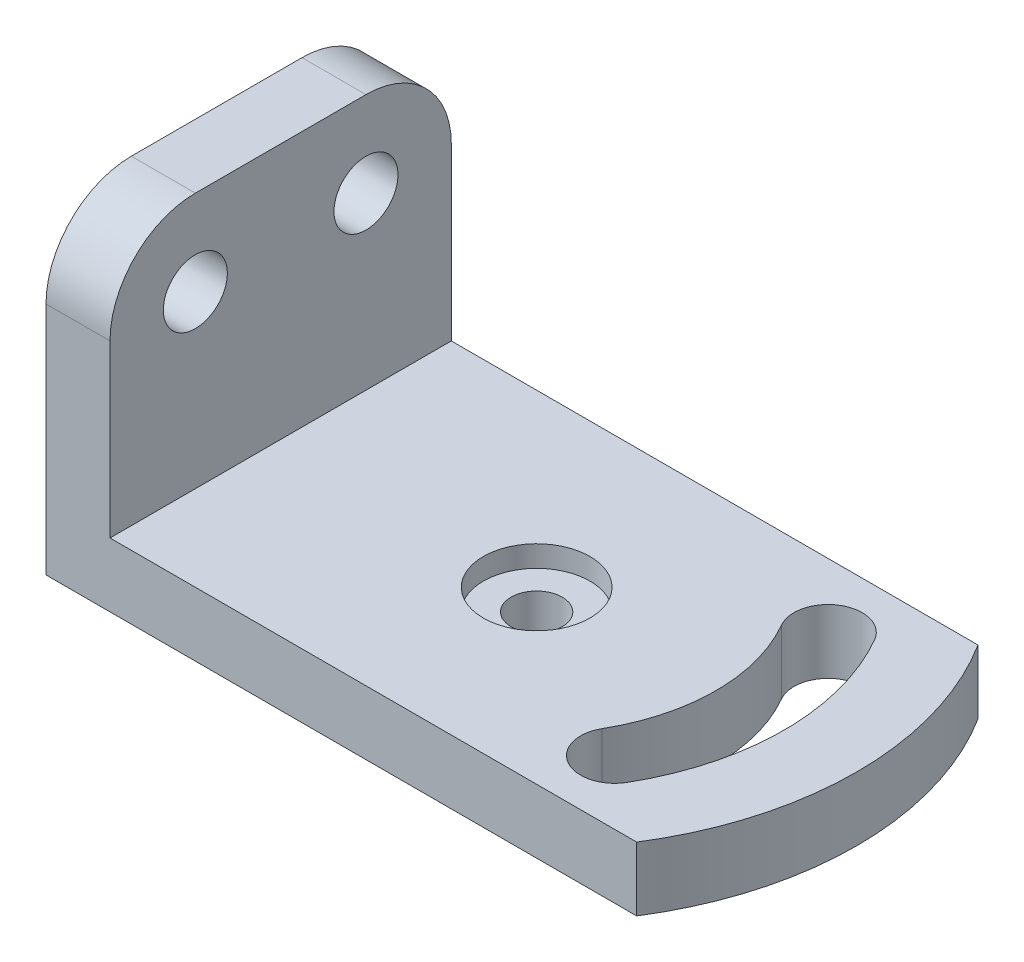
ISO-10303-21;
HEADER;
FILE_DESCRIPTION(('STEP AP214'),'2;1');
FILE_NAME('part.step','',(''),(''),'','','');
FILE_SCHEMA(('AUTOMOTIVE_DESIGN { 1 0 10303 214 1 1 1 1 }'));
ENDSEC;
DATA;
#1=APPLICATION_CONTEXT('core data for automotive mechanical design processes');
#2=APPLICATION_PROTOCOL_DEFINITION('international standard','automotive_design',2000,#1);
#3=PRODUCT_CONTEXT('',#1,'mechanical');
#4=PRODUCT('Part','Part','',(#3));
#5=PRODUCT_RELATED_PRODUCT_CATEGORY('part','',(#4));
#6=PRODUCT_DEFINITION_FORMATION('','',#4);
#7=PRODUCT_DEFINITION_CONTEXT('part definition',#1,'design');
#8=PRODUCT_DEFINITION('design','',#6,#7);
#9=PRODUCT_DEFINITION_SHAPE('','',#8);
#10=(LENGTH_UNIT() NAMED_UNIT(*) SI_UNIT(.MILLI.,.METRE.));
#11=(NAMED_UNIT(*) PLANE_ANGLE_UNIT() SI_UNIT($,.RADIAN.));
#12=(NAMED_UNIT(*) SI_UNIT($,.STERADIAN.) SOLID_ANGLE_UNIT());
#13=UNCERTAINTY_MEASURE_WITH_UNIT(LENGTH_MEASURE(1.E-05),#10,'distance_accuracy_value','');
#14=(GEOMETRIC_REPRESENTATION_CONTEXT(3) GLOBAL_UNCERTAINTY_ASSIGNED_CONTEXT((#13)) GLOBAL_UNIT_ASSIGNED_CONTEXT((#10,
#11,#12)) REPRESENTATION_CONTEXT('',''));
#15=CARTESIAN_POINT('',(0.,0.,0.));
#16=DIRECTION('',(0.,0.,1.));
#17=DIRECTION('',(1.,0.,0.));
#18=AXIS2_PLACEMENT_3D('',#15,#16,#17);
#19=CARTESIAN_POINT('',(0.,15.,0.));
#20=DIRECTION('',(0.,1.,0.));
#21=DIRECTION('',(0.,0.,1.));
#22=AXIS2_PLACEMENT_3D('',#19,#20,#21);
#23=PLANE('',#22);
#24=CARTESIAN_POINT('',(43.3012701892219,15.,25.0000000000001));
#25=DIRECTION('',(0.,1.,0.));
#26=DIRECTION('',(0.,0.,1.));
#27=AXIS2_PLACEMENT_3D('',#24,#25,#26);
#28=CIRCLE('',#27,7.99999999999999);
#29=CARTESIAN_POINT('',(36.3730669589464,15.,21.));
#30=VERTEX_POINT('',#29);
#31=CARTESIAN_POINT('',(50.2294734194974,15.,29.0000000000001));
#32=VERTEX_POINT('',#31);
#33=EDGE_CURVE('E61',#30,#32,#28,.T.);
#34=ORIENTED_EDGE('',*,*,#33,.F.);
#35=CARTESIAN_POINT('',(0.,15.,0.));
#36=DIRECTION('',(0.,1.,0.));
#37=DIRECTION('',(0.,0.,1.));
#38=AXIS2_PLACEMENT_3D('',#35,#36,#37);
#39=CIRCLE('',#38,42.);
#40=CARTESIAN_POINT('',(36.3730669589464,15.,-21.0000000000001));
#41=VERTEX_POINT('',#40);
#42=EDGE_CURVE('E182',#30,#41,#39,.T.);
#43=ORIENTED_EDGE('',*,*,#42,.T.);
#44=CARTESIAN_POINT('',(43.3012701892219,15.,-25.0000000000001));
#45=DIRECTION('',(0.,1.,0.));
#46=DIRECTION('',(0.,0.,1.));
#47=AXIS2_PLACEMENT_3D('',#44,#45,#46);
#48=CIRCLE('',#47,7.99999999999999);
#49=CARTESIAN_POINT('',(50.2294734194974,15.,-29.0000000000001));
#50=VERTEX_POINT('',#49);
#51=EDGE_CURVE('E179',#50,#41,#48,.T.);
#52=ORIENTED_EDGE('',*,*,#51,.F.);
#53=CARTESIAN_POINT('',(0.,15.,0.));
#54=DIRECTION('',(0.,1.,0.));
#55=DIRECTION('',(0.,0.,1.));
#56=AXIS2_PLACEMENT_3D('',#53,#54,#55);
#57=CIRCLE('',#56,58.);
#58=EDGE_CURVE('E180',#32,#50,#57,.T.);
#59=ORIENTED_EDGE('',*,*,#58,.F.);
#60=EDGE_LOOP('',(#34,#43,#52,#59));
#61=FACE_BOUND('',#60,.T.);
#62=CARTESIAN_POINT('',(0.,15.,0.));
#63=DIRECTION('',(0.,1.,0.));
#64=DIRECTION('',(0.,0.,1.));
#65=AXIS2_PLACEMENT_3D('',#62,#63,#64);
#66=CIRCLE('',#65,12.5);
#67=CARTESIAN_POINT('',(0.,15.,12.5));
#68=VERTEX_POINT('',#67);
#69=EDGE_CURVE('E212',#68,#68,#66,.T.);
#70=ORIENTED_EDGE('',*,*,#69,.F.);
#71=EDGE_LOOP('',(#70));
#72=FACE_BOUND('',#71,.T.);
#73=DIRECTION('',(-1.,0.,0.));
#74=VECTOR('',#73,1.);
#75=CARTESIAN_POINT('',(-75.,15.,-40.));
#76=LINE('',#75,#74);
#77=CARTESIAN_POINT('',(63.4428877022476,15.,-40.));
#78=VERTEX_POINT('',#77);
#79=CARTESIAN_POINT('',(-60.,15.,-40.));
#80=VERTEX_POINT('',#79);
#81=EDGE_CURVE('E228',#78,#80,#76,.T.);
#82=ORIENTED_EDGE('',*,*,#81,.T.);
#83=DIRECTION('',(0.,0.,1.));
#84=VECTOR('',#83,1.);
#85=CARTESIAN_POINT('',(-60.,15.,-40.));
#86=LINE('',#85,#84);
#87=CARTESIAN_POINT('',(-60.,15.,40.));
#88=VERTEX_POINT('',#87);
#89=EDGE_CURVE('E165',#80,#88,#86,.T.);
#90=ORIENTED_EDGE('',*,*,#89,.T.);
#91=DIRECTION('',(1.,0.,0.));
#92=VECTOR('',#91,1.);
#93=CARTESIAN_POINT('',(-75.,15.,40.));
#94=LINE('',#93,#92);
#95=CARTESIAN_POINT('',(63.4428877022476,15.,40.));
#96=VERTEX_POINT('',#95);
#97=EDGE_CURVE('E230',#88,#96,#94,.T.);
#98=ORIENTED_EDGE('',*,*,#97,.T.);
#99=CARTESIAN_POINT('',(0.,15.,0.));
#100=DIRECTION('',(0.,1.,0.));
#101=DIRECTION('',(0.,0.,1.));
#102=AXIS2_PLACEMENT_3D('',#99,#100,#101);
#103=CIRCLE('',#102,75.);
#104=EDGE_CURVE('E217',#96,#78,#103,.T.);
#105=ORIENTED_EDGE('',*,*,#104,.T.);
#106=EDGE_LOOP('',(#82,#90,#98,#105));
#107=FACE_BOUND('',#106,.T.);
#108=ADVANCED_FACE('F41',(#61,#72,#107),#23,.T.);
#109=CARTESIAN_POINT('',(0.,0.,0.));
#110=DIRECTION('',(0.,1.,0.));
#111=DIRECTION('',(0.,0.,1.));
#112=AXIS2_PLACEMENT_3D('',#109,#110,#111);
#113=PLANE('',#112);
#114=CARTESIAN_POINT('',(0.,0.,0.));
#115=DIRECTION('',(0.,1.,0.));
#116=DIRECTION('',(0.,0.,1.));
#117=AXIS2_PLACEMENT_3D('',#114,#115,#116);
#118=CIRCLE('',#117,42.);
#119=CARTESIAN_POINT('',(36.3730669589464,0.,21.));
#120=VERTEX_POINT('',#119);
#121=CARTESIAN_POINT('',(36.3730669589464,0.,-21.0000000000001));
#122=VERTEX_POINT('',#121);
#123=EDGE_CURVE('E193',#120,#122,#118,.T.);
#124=ORIENTED_EDGE('',*,*,#123,.F.);
#125=CARTESIAN_POINT('',(43.3012701892219,0.,25.0000000000001));
#126=DIRECTION('',(0.,1.,0.));
#127=DIRECTION('',(0.,0.,1.));
#128=AXIS2_PLACEMENT_3D('',#125,#126,#127);
#129=CIRCLE('',#128,7.99999999999999);
#130=CARTESIAN_POINT('',(50.2294734194974,0.,29.0000000000001));
#131=VERTEX_POINT('',#130);
#132=EDGE_CURVE('E187',#120,#131,#129,.T.);
#133=ORIENTED_EDGE('',*,*,#132,.T.);
#134=CARTESIAN_POINT('',(0.,0.,0.));
#135=DIRECTION('',(0.,1.,0.));
#136=DIRECTION('',(0.,0.,1.));
#137=AXIS2_PLACEMENT_3D('',#134,#135,#136);
#138=CIRCLE('',#137,58.);
#139=CARTESIAN_POINT('',(50.2294734194974,0.,-29.0000000000001));
#140=VERTEX_POINT('',#139);
#141=EDGE_CURVE('E186',#131,#140,#138,.T.);
#142=ORIENTED_EDGE('',*,*,#141,.T.);
#143=CARTESIAN_POINT('',(43.3012701892219,0.,-25.0000000000001));
#144=DIRECTION('',(0.,1.,0.));
#145=DIRECTION('',(0.,0.,1.));
#146=AXIS2_PLACEMENT_3D('',#143,#144,#145);
#147=CIRCLE('',#146,7.99999999999999);
#148=EDGE_CURVE('E195',#140,#122,#147,.T.);
#149=ORIENTED_EDGE('',*,*,#148,.T.);
#150=EDGE_LOOP('',(#124,#133,#142,#149));
#151=FACE_BOUND('',#150,.T.);
#152=CARTESIAN_POINT('',(0.,0.,0.));
#153=DIRECTION('',(0.,1.,0.));
#154=DIRECTION('',(0.,0.,1.));
#155=AXIS2_PLACEMENT_3D('',#152,#153,#154);
#156=CIRCLE('',#155,6.);
#157=CARTESIAN_POINT('',(0.,0.,6.));
#158=VERTEX_POINT('',#157);
#159=EDGE_CURVE('E206',#158,#158,#156,.T.);
#160=ORIENTED_EDGE('',*,*,#159,.T.);
#161=EDGE_LOOP('',(#160));
#162=FACE_BOUND('',#161,.T.);
#163=CARTESIAN_POINT('',(0.,0.,0.));
#164=DIRECTION('',(0.,1.,0.));
#165=DIRECTION('',(0.,0.,1.));
#166=AXIS2_PLACEMENT_3D('',#163,#164,#165);
#167=CIRCLE('',#166,75.);
#168=CARTESIAN_POINT('',(63.4428877022476,0.,40.));
#169=VERTEX_POINT('',#168);
#170=CARTESIAN_POINT('',(63.4428877022476,0.,-40.));
#171=VERTEX_POINT('',#170);
#172=EDGE_CURVE('E11',#169,#171,#167,.T.);
#173=ORIENTED_EDGE('',*,*,#172,.F.);
#174=DIRECTION('',(1.,0.,0.));
#175=VECTOR('',#174,1.);
#176=CARTESIAN_POINT('',(-75.,0.,40.));
#177=LINE('',#176,#175);
#178=CARTESIAN_POINT('',(-75.,0.,40.));
#179=VERTEX_POINT('',#178);
#180=EDGE_CURVE('E229',#179,#169,#177,.T.);
#181=ORIENTED_EDGE('',*,*,#180,.F.);
#182=DIRECTION('',(0.,0.,1.));
#183=VECTOR('',#182,1.);
#184=CARTESIAN_POINT('',(-75.,0.,-40.));
#185=LINE('',#184,#183);
#186=CARTESIAN_POINT('',(-75.,0.,-40.));
#187=VERTEX_POINT('',#186);
#188=EDGE_CURVE('E234',#187,#179,#185,.T.);
#189=ORIENTED_EDGE('',*,*,#188,.F.);
#190=DIRECTION('',(-1.,0.,0.));
#191=VECTOR('',#190,1.);
#192=CARTESIAN_POINT('',(-75.,0.,-40.));
#193=LINE('',#192,#191);
#194=EDGE_CURVE('E221',#171,#187,#193,.T.);
#195=ORIENTED_EDGE('',*,*,#194,.F.);
#196=EDGE_LOOP('',(#173,#181,#189,#195));
#197=FACE_BOUND('',#196,.T.);
#198=ADVANCED_FACE('F248',(#151,#162,#197),#113,.F.);
#199=CARTESIAN_POINT('',(-75.,15.,-40.));
#200=DIRECTION('',(0.,0.,1.));
#201=DIRECTION('',(1.,0.,0.));
#202=AXIS2_PLACEMENT_3D('',#199,#200,#201);
#203=PLANE('',#202);
#204=DIRECTION('',(0.,1.,0.));
#205=VECTOR('',#204,1.);
#206=CARTESIAN_POINT('',(63.4428877022476,-20.,-40.));
#207=LINE('',#206,#205);
#208=EDGE_CURVE('E222',#171,#78,#207,.T.);
#209=ORIENTED_EDGE('',*,*,#208,.F.);
#210=ORIENTED_EDGE('',*,*,#194,.T.);
#211=DIRECTION('',(0.,-1.,0.));
#212=VECTOR('',#211,1.);
#213=CARTESIAN_POINT('',(-75.,15.,-40.));
#214=LINE('',#213,#212);
#215=CARTESIAN_POINT('',(-75.,54.9999999999999,-40.));
#216=VERTEX_POINT('',#215);
#217=EDGE_CURVE('E47',#216,#187,#214,.T.);
#218=ORIENTED_EDGE('',*,*,#217,.F.);
#219=DIRECTION('',(-1.,0.,0.));
#220=VECTOR('',#219,1.);
#221=CARTESIAN_POINT('',(-60.,54.9999999999999,-40.));
#222=LINE('',#221,#220);
#223=CARTESIAN_POINT('',(-60.,54.9999999999999,-40.));
#224=VERTEX_POINT('',#223);
#225=EDGE_CURVE('E175',#224,#216,#222,.T.);
#226=ORIENTED_EDGE('',*,*,#225,.F.);
#227=DIRECTION('',(0.,-1.,0.));
#228=VECTOR('',#227,1.);
#229=CARTESIAN_POINT('',(-60.,15.,-40.));
#230=LINE('',#229,#228);
#231=EDGE_CURVE('E163',#224,#80,#230,.T.);
#232=ORIENTED_EDGE('',*,*,#231,.T.);
#233=ORIENTED_EDGE('',*,*,#81,.F.);
#234=EDGE_LOOP('',(#209,#210,#218,#226,#232,#233));
#235=FACE_BOUND('',#234,.T.);
#236=ADVANCED_FACE('F43',(#235),#203,.F.);
#237=CARTESIAN_POINT('',(-75.,15.,-40.));
#238=DIRECTION('',(1.,0.,0.));
#239=DIRECTION('',(0.,0.,-1.));
#240=AXIS2_PLACEMENT_3D('',#237,#238,#239);
#241=PLANE('',#240);
#242=ORIENTED_EDGE('',*,*,#188,.T.);
#243=DIRECTION('',(0.,-1.,0.));
#244=VECTOR('',#243,1.);
#245=CARTESIAN_POINT('',(-75.,15.,40.));
#246=LINE('',#245,#244);
#247=CARTESIAN_POINT('',(-75.,54.9999999999999,40.));
#248=VERTEX_POINT('',#247);
#249=EDGE_CURVE('E235',#248,#179,#246,.T.);
#250=ORIENTED_EDGE('',*,*,#249,.F.);
#251=CARTESIAN_POINT('',(-75.,55.,20.));
#252=DIRECTION('',(-1.,0.,0.));
#253=DIRECTION('',(0.,0.,-1.));
#254=AXIS2_PLACEMENT_3D('',#251,#252,#253);
#255=CIRCLE('',#254,20.);
#256=CARTESIAN_POINT('',(-75.,75.,19.9999999999999));
#257=VERTEX_POINT('',#256);
#258=EDGE_CURVE('E170',#248,#257,#255,.T.);
#259=ORIENTED_EDGE('',*,*,#258,.T.);
#260=DIRECTION('',(0.,0.,-1.));
#261=VECTOR('',#260,1.);
#262=CARTESIAN_POINT('',(-75.,75.,-19.9999999999999));
#263=LINE('',#262,#261);
#264=CARTESIAN_POINT('',(-75.,75.,-19.9999999999999));
#265=VERTEX_POINT('',#264);
#266=EDGE_CURVE('E132',#257,#265,#263,.T.);
#267=ORIENTED_EDGE('',*,*,#266,.T.);
#268=CARTESIAN_POINT('',(-75.,55.,-20.));
#269=DIRECTION('',(-1.,0.,0.));
#270=DIRECTION('',(0.,0.,-1.));
#271=AXIS2_PLACEMENT_3D('',#268,#269,#270);
#272=CIRCLE('',#271,20.);
#273=EDGE_CURVE('E151',#265,#216,#272,.T.);
#274=ORIENTED_EDGE('',*,*,#273,.T.);
#275=ORIENTED_EDGE('',*,*,#217,.T.);
#276=EDGE_LOOP('',(#242,#250,#259,#267,#274,#275));
#277=FACE_BOUND('',#276,.T.);
#278=CARTESIAN_POINT('',(-75.,55.,20.));
#279=DIRECTION('',(-1.,0.,0.));
#280=DIRECTION('',(0.,0.,1.));
#281=AXIS2_PLACEMENT_3D('',#278,#279,#280);
#282=CIRCLE('',#281,7.5);
#283=CARTESIAN_POINT('',(-75.,55.,27.5));
#284=VERTEX_POINT('',#283);
#285=EDGE_CURVE('E366',#284,#284,#282,.T.);
#286=ORIENTED_EDGE('',*,*,#285,.F.);
#287=EDGE_LOOP('',(#286));
#288=FACE_BOUND('',#287,.T.);
#289=CARTESIAN_POINT('',(-75.,55.,-20.));
#290=DIRECTION('',(-1.,0.,0.));
#291=DIRECTION('',(0.,0.,1.));
#292=AXIS2_PLACEMENT_3D('',#289,#290,#291);
#293=CIRCLE('',#292,7.5);
#294=CARTESIAN_POINT('',(-75.,55.,-12.5));
#295=VERTEX_POINT('',#294);
#296=EDGE_CURVE('E159',#295,#295,#293,.T.);
#297=ORIENTED_EDGE('',*,*,#296,.F.);
#298=EDGE_LOOP('',(#297));
#299=FACE_BOUND('',#298,.T.);
#300=ADVANCED_FACE('F245',(#277,#288,#299),#241,.F.);
#301=CARTESIAN_POINT('',(-75.,15.,40.));
#302=DIRECTION('',(0.,0.,-1.));
#303=DIRECTION('',(-1.,0.,0.));
#304=AXIS2_PLACEMENT_3D('',#301,#302,#303);
#305=PLANE('',#304);
#306=ORIENTED_EDGE('',*,*,#180,.T.);
#307=DIRECTION('',(0.,1.,0.));
#308=VECTOR('',#307,1.);
#309=CARTESIAN_POINT('',(63.4428877022476,-20.,40.));
#310=LINE('',#309,#308);
#311=EDGE_CURVE('E213',#169,#96,#310,.T.);
#312=ORIENTED_EDGE('',*,*,#311,.T.);
#313=ORIENTED_EDGE('',*,*,#97,.F.);
#314=DIRECTION('',(0.,1.,0.));
#315=VECTOR('',#314,1.);
#316=CARTESIAN_POINT('',(-60.,15.,40.));
#317=LINE('',#316,#315);
#318=CARTESIAN_POINT('',(-60.,54.9999999999999,40.));
#319=VERTEX_POINT('',#318);
#320=EDGE_CURVE('E57',#88,#319,#317,.T.);
#321=ORIENTED_EDGE('',*,*,#320,.T.);
#322=DIRECTION('',(-1.,0.,0.));
#323=VECTOR('',#322,1.);
#324=CARTESIAN_POINT('',(-60.,54.9999999999999,40.));
#325=LINE('',#324,#323);
#326=EDGE_CURVE('E154',#319,#248,#325,.T.);
#327=ORIENTED_EDGE('',*,*,#326,.T.);
#328=ORIENTED_EDGE('',*,*,#249,.T.);
#329=EDGE_LOOP('',(#306,#312,#313,#321,#327,#328));
#330=FACE_BOUND('',#329,.T.);
#331=ADVANCED_FACE('F255',(#330),#305,.F.);
#332=CARTESIAN_POINT('',(0.,-20.,0.));
#333=DIRECTION('',(0.,1.,0.));
#334=DIRECTION('',(0.,0.,1.));
#335=AXIS2_PLACEMENT_3D('',#332,#333,#334);
#336=CYLINDRICAL_SURFACE('',#335,75.);
#337=ORIENTED_EDGE('',*,*,#172,.T.);
#338=ORIENTED_EDGE('',*,*,#208,.T.);
#339=ORIENTED_EDGE('',*,*,#104,.F.);
#340=ORIENTED_EDGE('',*,*,#311,.F.);
#341=EDGE_LOOP('',(#337,#338,#339,#340));
#342=FACE_BOUND('',#341,.T.);
#343=ADVANCED_FACE('F259',(#342),#336,.T.);
#344=CARTESIAN_POINT('',(0.,10.,0.));
#345=DIRECTION('',(0.,1.,0.));
#346=DIRECTION('',(0.,0.,1.));
#347=AXIS2_PLACEMENT_3D('',#344,#345,#346);
#348=CYLINDRICAL_SURFACE('',#347,12.5);
#349=CARTESIAN_POINT('',(0.,10.,0.));
#350=DIRECTION('',(0.,1.,0.));
#351=DIRECTION('',(0.,0.,1.));
#352=AXIS2_PLACEMENT_3D('',#349,#350,#351);
#353=CIRCLE('',#352,12.5);
#354=CARTESIAN_POINT('',(0.,10.,12.5));
#355=VERTEX_POINT('',#354);
#356=EDGE_CURVE('E215',#355,#355,#353,.T.);
#357=ORIENTED_EDGE('',*,*,#356,.F.);
#358=EDGE_LOOP('',(#357));
#359=FACE_BOUND('',#358,.T.);
#360=ORIENTED_EDGE('',*,*,#69,.T.);
#361=EDGE_LOOP('',(#360));
#362=FACE_BOUND('',#361,.T.);
#363=ADVANCED_FACE('F425',(#359,#362),#348,.F.);
#364=CARTESIAN_POINT('',(0.,10.,0.));
#365=DIRECTION('',(0.,1.,0.));
#366=DIRECTION('',(0.,0.,1.));
#367=AXIS2_PLACEMENT_3D('',#364,#365,#366);
#368=PLANE('',#367);
#369=CARTESIAN_POINT('',(0.,10.,0.));
#370=DIRECTION('',(0.,1.,0.));
#371=DIRECTION('',(0.,0.,1.));
#372=AXIS2_PLACEMENT_3D('',#369,#370,#371);
#373=CIRCLE('',#372,6.);
#374=CARTESIAN_POINT('',(0.,10.,6.));
#375=VERTEX_POINT('',#374);
#376=EDGE_CURVE('E197',#375,#375,#373,.T.);
#377=ORIENTED_EDGE('',*,*,#376,.F.);
#378=EDGE_LOOP('',(#377));
#379=FACE_BOUND('',#378,.T.);
#380=ORIENTED_EDGE('',*,*,#356,.T.);
#381=EDGE_LOOP('',(#380));
#382=FACE_BOUND('',#381,.T.);
#383=ADVANCED_FACE('F412',(#379,#382),#368,.T.);
#384=CARTESIAN_POINT('',(0.,-10.,0.));
#385=DIRECTION('',(0.,1.,0.));
#386=DIRECTION('',(0.,0.,1.));
#387=AXIS2_PLACEMENT_3D('',#384,#385,#386);
#388=CYLINDRICAL_SURFACE('',#387,6.);
#389=ORIENTED_EDGE('',*,*,#376,.T.);
#390=EDGE_LOOP('',(#389));
#391=FACE_BOUND('',#390,.T.);
#392=ORIENTED_EDGE('',*,*,#159,.F.);
#393=EDGE_LOOP('',(#392));
#394=FACE_BOUND('',#393,.T.);
#395=ADVANCED_FACE('F410',(#391,#394),#388,.F.);
#396=CARTESIAN_POINT('',(43.3012701892219,0.,25.0000000000001));
#397=DIRECTION('',(0.,1.,0.));
#398=DIRECTION('',(0.,0.,1.));
#399=AXIS2_PLACEMENT_3D('',#396,#397,#398);
#400=CYLINDRICAL_SURFACE('',#399,7.99999999999999);
#401=DIRECTION('',(0.,1.,0.));
#402=VECTOR('',#401,1.);
#403=CARTESIAN_POINT('',(50.2294734194974,0.,29.0000000000001));
#404=LINE('',#403,#402);
#405=EDGE_CURVE('E196',#131,#32,#404,.T.);
#406=ORIENTED_EDGE('',*,*,#405,.F.);
#407=ORIENTED_EDGE('',*,*,#132,.F.);
#408=DIRECTION('',(0.,1.,0.));
#409=VECTOR('',#408,1.);
#410=CARTESIAN_POINT('',(36.3730669589464,0.,21.));
#411=LINE('',#410,#409);
#412=EDGE_CURVE('E200',#120,#30,#411,.T.);
#413=ORIENTED_EDGE('',*,*,#412,.T.);
#414=ORIENTED_EDGE('',*,*,#33,.T.);
#415=EDGE_LOOP('',(#406,#407,#413,#414));
#416=FACE_BOUND('',#415,.T.);
#417=ADVANCED_FACE('F397',(#416),#400,.F.);
#418=CARTESIAN_POINT('',(0.,0.,0.));
#419=DIRECTION('',(0.,1.,0.));
#420=DIRECTION('',(0.,0.,1.));
#421=AXIS2_PLACEMENT_3D('',#418,#419,#420);
#422=CYLINDRICAL_SURFACE('',#421,42.);
#423=ORIENTED_EDGE('',*,*,#412,.F.);
#424=ORIENTED_EDGE('',*,*,#123,.T.);
#425=DIRECTION('',(0.,1.,0.));
#426=VECTOR('',#425,1.);
#427=CARTESIAN_POINT('',(36.3730669589464,0.,-21.0000000000001));
#428=LINE('',#427,#426);
#429=EDGE_CURVE('E203',#122,#41,#428,.T.);
#430=ORIENTED_EDGE('',*,*,#429,.T.);
#431=ORIENTED_EDGE('',*,*,#42,.F.);
#432=EDGE_LOOP('',(#423,#424,#430,#431));
#433=FACE_BOUND('',#432,.T.);
#434=ADVANCED_FACE('F386',(#433),#422,.T.);
#435=CARTESIAN_POINT('',(43.3012701892219,0.,-25.0000000000001));
#436=DIRECTION('',(0.,1.,0.));
#437=DIRECTION('',(0.,0.,1.));
#438=AXIS2_PLACEMENT_3D('',#435,#436,#437);
#439=CYLINDRICAL_SURFACE('',#438,7.99999999999999);
#440=ORIENTED_EDGE('',*,*,#429,.F.);
#441=ORIENTED_EDGE('',*,*,#148,.F.);
#442=DIRECTION('',(0.,1.,0.));
#443=VECTOR('',#442,1.);
#444=CARTESIAN_POINT('',(50.2294734194974,0.,-29.0000000000001));
#445=LINE('',#444,#443);
#446=EDGE_CURVE('E202',#140,#50,#445,.T.);
#447=ORIENTED_EDGE('',*,*,#446,.T.);
#448=ORIENTED_EDGE('',*,*,#51,.T.);
#449=EDGE_LOOP('',(#440,#441,#447,#448));
#450=FACE_BOUND('',#449,.T.);
#451=ADVANCED_FACE('F379',(#450),#439,.F.);
#452=CARTESIAN_POINT('',(0.,0.,0.));
#453=DIRECTION('',(0.,1.,0.));
#454=DIRECTION('',(0.,0.,1.));
#455=AXIS2_PLACEMENT_3D('',#452,#453,#454);
#456=CYLINDRICAL_SURFACE('',#455,58.);
#457=ORIENTED_EDGE('',*,*,#446,.F.);
#458=ORIENTED_EDGE('',*,*,#141,.F.);
#459=ORIENTED_EDGE('',*,*,#405,.T.);
#460=ORIENTED_EDGE('',*,*,#58,.T.);
#461=EDGE_LOOP('',(#457,#458,#459,#460));
#462=FACE_BOUND('',#461,.T.);
#463=ADVANCED_FACE('F270',(#462),#456,.F.);
#464=CARTESIAN_POINT('',(-60.,55.,20.));
#465=DIRECTION('',(-1.,0.,0.));
#466=DIRECTION('',(0.,0.,1.));
#467=AXIS2_PLACEMENT_3D('',#464,#465,#466);
#468=CYLINDRICAL_SURFACE('',#467,20.);
#469=ORIENTED_EDGE('',*,*,#258,.F.);
#470=ORIENTED_EDGE('',*,*,#326,.F.);
#471=CARTESIAN_POINT('',(-60.,55.,20.));
#472=DIRECTION('',(-1.,0.,0.));
#473=DIRECTION('',(0.,0.,-1.));
#474=AXIS2_PLACEMENT_3D('',#471,#472,#473);
#475=CIRCLE('',#474,20.);
#476=CARTESIAN_POINT('',(-60.,75.,19.9999999999999));
#477=VERTEX_POINT('',#476);
#478=EDGE_CURVE('E144',#319,#477,#475,.T.);
#479=ORIENTED_EDGE('',*,*,#478,.T.);
#480=DIRECTION('',(-1.,0.,0.));
#481=VECTOR('',#480,1.);
#482=CARTESIAN_POINT('',(-60.,75.,19.9999999999999));
#483=LINE('',#482,#481);
#484=EDGE_CURVE('E128',#477,#257,#483,.T.);
#485=ORIENTED_EDGE('',*,*,#484,.T.);
#486=EDGE_LOOP('',(#469,#470,#479,#485));
#487=FACE_BOUND('',#486,.T.);
#488=ADVANCED_FACE('F146',(#487),#468,.T.);
#489=CARTESIAN_POINT('',(-60.,55.,-20.));
#490=DIRECTION('',(-1.,0.,0.));
#491=DIRECTION('',(0.,0.,1.));
#492=AXIS2_PLACEMENT_3D('',#489,#490,#491);
#493=CYLINDRICAL_SURFACE('',#492,20.);
#494=ORIENTED_EDGE('',*,*,#273,.F.);
#495=DIRECTION('',(-1.,0.,0.));
#496=VECTOR('',#495,1.);
#497=CARTESIAN_POINT('',(-60.,75.,-19.9999999999999));
#498=LINE('',#497,#496);
#499=CARTESIAN_POINT('',(-60.,75.,-19.9999999999999));
#500=VERTEX_POINT('',#499);
#501=EDGE_CURVE('E136',#500,#265,#498,.T.);
#502=ORIENTED_EDGE('',*,*,#501,.F.);
#503=CARTESIAN_POINT('',(-60.,55.,-20.));
#504=DIRECTION('',(-1.,0.,0.));
#505=DIRECTION('',(0.,0.,-1.));
#506=AXIS2_PLACEMENT_3D('',#503,#504,#505);
#507=CIRCLE('',#506,20.);
#508=EDGE_CURVE('E150',#500,#224,#507,.T.);
#509=ORIENTED_EDGE('',*,*,#508,.T.);
#510=ORIENTED_EDGE('',*,*,#225,.T.);
#511=EDGE_LOOP('',(#494,#502,#509,#510));
#512=FACE_BOUND('',#511,.T.);
#513=ADVANCED_FACE('F264',(#512),#493,.T.);
#514=CARTESIAN_POINT('',(-60.,75.,-19.9999999999999));
#515=DIRECTION('',(0.,1.,0.));
#516=DIRECTION('',(0.,0.,1.));
#517=AXIS2_PLACEMENT_3D('',#514,#515,#516);
#518=PLANE('',#517);
#519=ORIENTED_EDGE('',*,*,#266,.F.);
#520=ORIENTED_EDGE('',*,*,#484,.F.);
#521=DIRECTION('',(0.,0.,-1.));
#522=VECTOR('',#521,1.);
#523=CARTESIAN_POINT('',(-60.,75.,-19.9999999999999));
#524=LINE('',#523,#522);
#525=EDGE_CURVE('E135',#477,#500,#524,.T.);
#526=ORIENTED_EDGE('',*,*,#525,.T.);
#527=ORIENTED_EDGE('',*,*,#501,.T.);
#528=EDGE_LOOP('',(#519,#520,#526,#527));
#529=FACE_BOUND('',#528,.T.);
#530=ADVANCED_FACE('F131',(#529),#518,.T.);
#531=CARTESIAN_POINT('',(-60.,55.,20.));
#532=DIRECTION('',(1.,0.,0.));
#533=DIRECTION('',(0.,0.,-1.));
#534=AXIS2_PLACEMENT_3D('',#531,#532,#533);
#535=PLANE('',#534);
#536=CARTESIAN_POINT('',(-60.,55.,20.));
#537=DIRECTION('',(-1.,0.,0.));
#538=DIRECTION('',(0.,0.,1.));
#539=AXIS2_PLACEMENT_3D('',#536,#537,#538);
#540=CIRCLE('',#539,7.5);
#541=CARTESIAN_POINT('',(-60.,55.,27.5));
#542=VERTEX_POINT('',#541);
#543=EDGE_CURVE('E361',#542,#542,#540,.T.);
#544=ORIENTED_EDGE('',*,*,#543,.T.);
#545=EDGE_LOOP('',(#544));
#546=FACE_BOUND('',#545,.T.);
#547=CARTESIAN_POINT('',(-60.,55.,-20.));
#548=DIRECTION('',(-1.,0.,0.));
#549=DIRECTION('',(0.,0.,1.));
#550=AXIS2_PLACEMENT_3D('',#547,#548,#549);
#551=CIRCLE('',#550,7.5);
#552=CARTESIAN_POINT('',(-60.,55.,-12.5));
#553=VERTEX_POINT('',#552);
#554=EDGE_CURVE('E169',#553,#553,#551,.T.);
#555=ORIENTED_EDGE('',*,*,#554,.T.);
#556=EDGE_LOOP('',(#555));
#557=FACE_BOUND('',#556,.T.);
#558=ORIENTED_EDGE('',*,*,#478,.F.);
#559=ORIENTED_EDGE('',*,*,#320,.F.);
#560=ORIENTED_EDGE('',*,*,#89,.F.);
#561=ORIENTED_EDGE('',*,*,#231,.F.);
#562=ORIENTED_EDGE('',*,*,#508,.F.);
#563=ORIENTED_EDGE('',*,*,#525,.F.);
#564=EDGE_LOOP('',(#558,#559,#560,#561,#562,#563));
#565=FACE_BOUND('',#564,.T.);
#566=ADVANCED_FACE('F141',(#546,#557,#565),#535,.T.);
#567=CARTESIAN_POINT('',(-60.,55.,-20.));
#568=DIRECTION('',(-1.,0.,0.));
#569=DIRECTION('',(0.,0.,1.));
#570=AXIS2_PLACEMENT_3D('',#567,#568,#569);
#571=CYLINDRICAL_SURFACE('',#570,7.5);
#572=ORIENTED_EDGE('',*,*,#554,.F.);
#573=EDGE_LOOP('',(#572));
#574=FACE_BOUND('',#573,.T.);
#575=ORIENTED_EDGE('',*,*,#296,.T.);
#576=EDGE_LOOP('',(#575));
#577=FACE_BOUND('',#576,.T.);
#578=ADVANCED_FACE('F336',(#574,#577),#571,.F.);
#579=CARTESIAN_POINT('',(-60.,55.,20.));
#580=DIRECTION('',(-1.,0.,0.));
#581=DIRECTION('',(0.,0.,1.));
#582=AXIS2_PLACEMENT_3D('',#579,#580,#581);
#583=CYLINDRICAL_SURFACE('',#582,7.5);
#584=ORIENTED_EDGE('',*,*,#543,.F.);
#585=EDGE_LOOP('',(#584));
#586=FACE_BOUND('',#585,.T.);
#587=ORIENTED_EDGE('',*,*,#285,.T.);
#588=EDGE_LOOP('',(#587));
#589=FACE_BOUND('',#588,.T.);
#590=ADVANCED_FACE('F346',(#586,#589),#583,.F.);
#591=CLOSED_SHELL('',(#108,#198,#236,#300,#331,#343,#363,#383,#395,#417,#434,#451,#463,#488,
#513,#530,#566,#578,#590));
#592=MANIFOLD_SOLID_BREP('B2',#591);
#593=ADVANCED_BREP_SHAPE_REPRESENTATION('',(#18,#592),#14);
#594=SHAPE_DEFINITION_REPRESENTATION(#9,#593);
ENDSEC;
END-ISO-10303-21;
